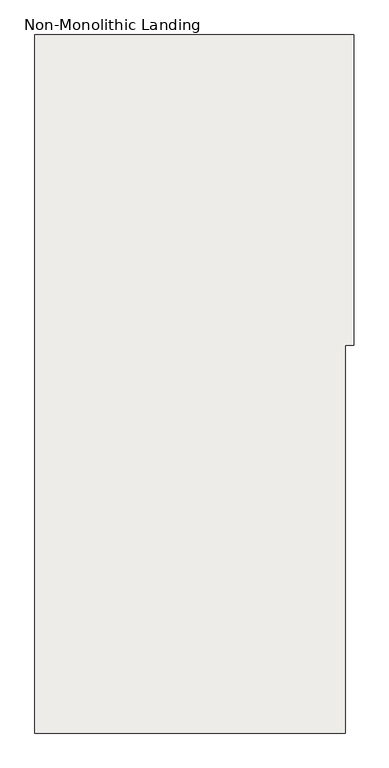
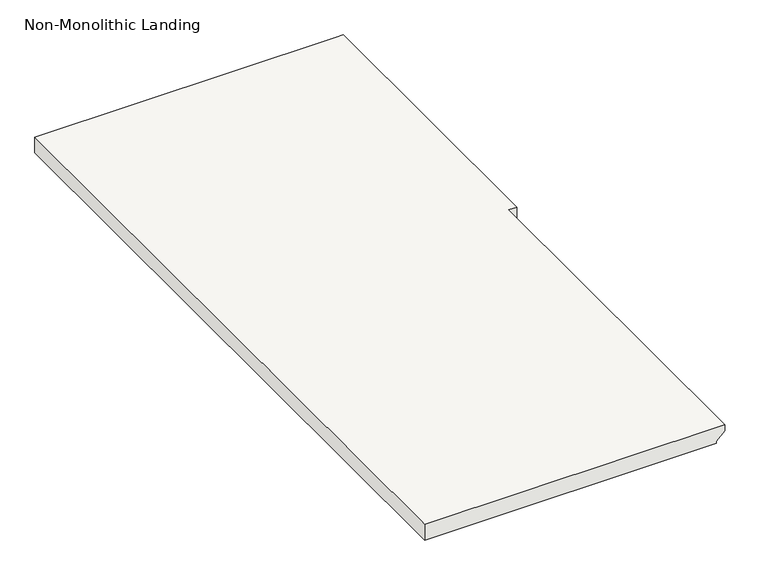
"""IFC4 building model written with IfcOpenShell, lengths in millimetres: slab geometry, Non-Monolithic Landing."""

from ifc_helpers import new_model, si_unit, origin, place, context, project, spatial, faceted_brep, source, transform, mapped, element, save


def non_monolithic_landing_0199e9fe(model_context):
    return source(origin(), model_context, "Body", "Brep", [
        faceted_brep([(-14575.9777023, -354.9320925, 4688.4166667), (-14601.3777023, -354.9320925, 4663.0166667), (-14601.3777023, 559.4679075, 4663.0166667), (-14575.9777023, 559.4679075, 4688.4166667), (-14575.9777023, 788.0679075, 4707.4666667), (-14550.5777023, 788.0679075, 4707.4666667), (-14550.5777023, 1702.4679075, 4707.4666667), (-14575.9777023, 1702.4679075, 4707.4666667), (-15490.3777023, 1702.4679075, 4707.4666667), (-15490.3777023, -354.9320925, 4707.4666667), (-14575.9777023, -354.9320925, 4707.4666667), (-14601.3777023, 559.4679075, 4656.6666667), (-14601.3777023, -354.9320925, 4656.6666667), (-15490.3777023, -354.9320925, 4656.6666667), (-15490.3777023, 1702.4679075, 4656.6666667), (-14575.9777023, 1702.4679075, 4656.6666667), (-14550.5777023, 1702.4679075, 4656.6666667), (-14550.5777023, 788.0679075, 4656.6666667), (-14575.9777023, 788.0679075, 4656.6666667), (-14575.9777023, 559.4679075, 4656.6666667)], [[[0, 1, 2, 3]], [[4, 5, 6, 7, 8, 9, 10]], [[11, 12, 13, 14, 15, 16, 17, 18, 19]], [[12, 11, 2, 1]], [[11, 19, 3, 2]], [[4, 10, 0, 3, 19, 18]], [[5, 4, 18, 17]], [[6, 5, 17, 16]], [[7, 6, 16, 15]], [[8, 7, 15, 14]], [[9, 8, 14, 13]], [[10, 9, 13, 12, 1, 0]]]),
    ])


if __name__ == "__main__":
    model = new_model("IFC4")
    model_context = context("Model", 3, world=origin())
    ifc_project = project(units=[si_unit("LENGTHUNIT", "METRE", prefix="MILLI")], contexts=[model_context])
    site = spatial("IfcSite", under=ifc_project)
    building = spatial("IfcBuilding", under=site)
    placement = place(None, origin())
    non_monolithic_landing_shape = non_monolithic_landing_0199e9fe(model_context)
    element("IfcSlab", 1, ObjectType="Non-Monolithic Landing", at=placement, inside=building, context=model_context, shape_type="MappedRepresentation", body=[
        mapped(non_monolithic_landing_shape, transform((0.0, 0.0, 0.0), x_axis=(1.0, 0.0, 0.0), y_axis=(0.0, 1.0, 0.0), z_axis=(0.0, 0.0, 1.0))),
    ])
    save(model, "model.ifc")
